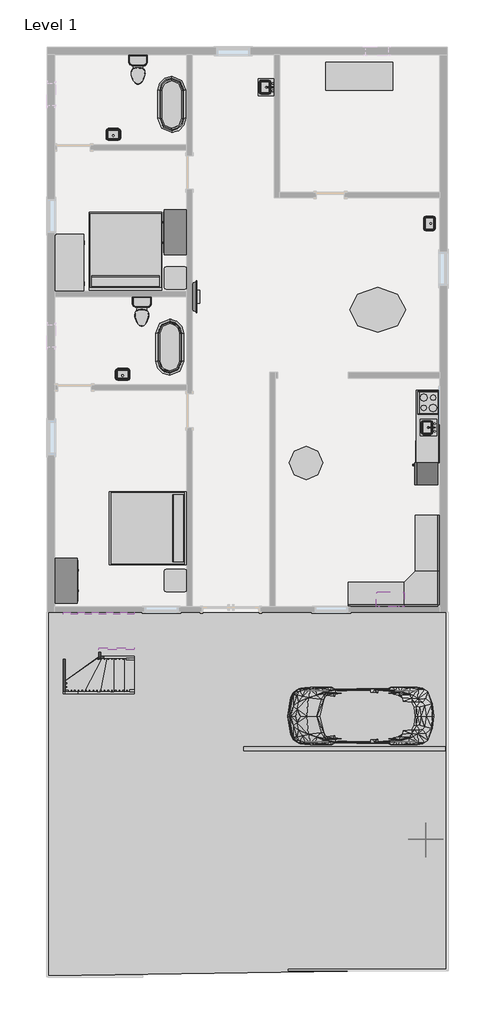
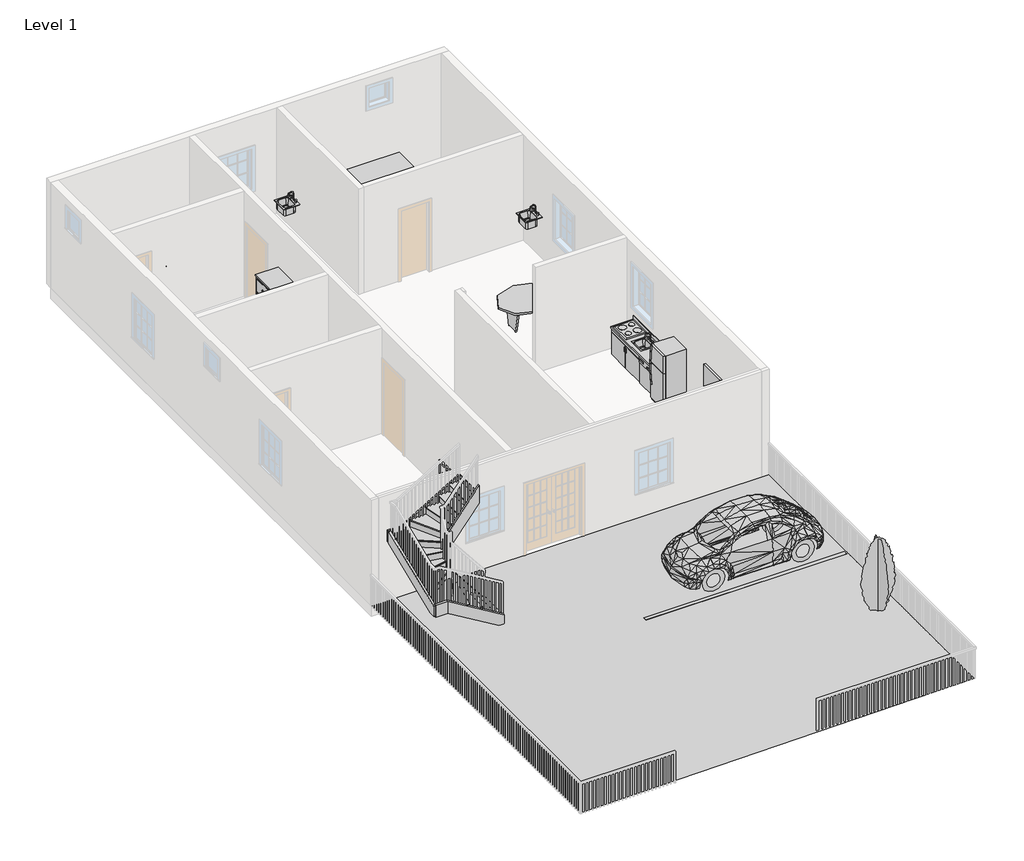
# One storey, part 5 of 5: 13 furniture elements, 9 flow terminals, 8 members, 8 proxies, 1 geographic element, 1 stair flight.
"""IFC4 building model written with IfcOpenShell, lengths in millimetres."""

from ifc_helpers import new_model, si_unit, frame, origin, place, context, project, spatial, polyline, outline, extrude, triangles, transform, mapped, element, save
from components import proxy_a6faaae8, proxy_45b28599, kitchenette_medium_kitchenette_medium_844211aa, proxy_8a8d5ab2, parking_space_9_x_18_90_deg_b8b21359, rpc_beetle_rpc_beetle_3ce7ba48, proxy_c523a7b7, flow_terminal_871c2e40, toilet_domestic_3d_toilet_domestic_3d_f7549cf7, toilet_domestic_3d_toilet_domestic_3d_183bbd19, flow_terminal_b374fae2, flow_terminal_f2f0329d, furniture_29cd36cd, furniture_c6510c7c, furniture_013ab306, furniture_9fa109b2, furniture_56245f3a, furniture_905aceb5, furniture_743965d2, furniture_bcf351fa, furniture_a5b052b6, furniture_45e3acac, rpc_tree_conifer_chinese_juniper_7_1b9786cd, stair_flight_9fd4ca1a

model = new_model("IFC4")

# Units and contexts
model_context = context("Model", 3, world=origin())
ifc_project = project(units=[si_unit("LENGTHUNIT", "METRE", prefix="MILLI")], contexts=[model_context])

# Site, building, storey
site = spatial("IfcSite", under=ifc_project)
building = spatial("IfcBuilding", under=site)
storey = spatial("IfcBuildingStorey", under=building, Name="Level 1", Elevation=0.0)

# Proxies
placement = place(None, origin())
element("IfcBuildingElementProxy", 1, Name="Building Element Proxy", at=placement, inside=storey, context=model_context, shape_type="Tessellation", body=[
    triangles([(-8987.0171402, -2473.4077469, 0.0), (-8987.0171402, -12354.0075531, 0.0), (1849.2579082, -12201.6075531, 0.0), (1833.3830051, -2473.4077469, 0.0)], [[1, 2, 3], [3, 4, 1]], closed=False),
])
proxy_shape = proxy_a6faaae8(model_context)
element("IfcBuildingElementProxy", 2, Name="Cook Top-4 Unit2 : 22\" x 20\"", ObjectType="Cook Top-4 Unit2 : 22\" x 20\"", at=placement, inside=storey, context=model_context, shape_type="MappedRepresentation", body=[
    mapped(proxy_shape, transform((1350.7829734, 3228.8923354, 0.0), x_axis=(0.0, -1.0000000000000004, 0.0), y_axis=(1.0000000000000004, 0.0, 0.0), z_axis=(0.0, 0.0, 1.0))),
])
proxy_2_shape = proxy_45b28599(model_context)
element("IfcBuildingElementProxy", 3, Name="Dishwasher : 24\" x 24\" x 34\"", ObjectType="Dishwasher : 24\" x 24\" x 34\"", at=placement, inside=storey, context=model_context, shape_type="MappedRepresentation", body=[
    mapped(proxy_2_shape, transform((1058.9334086, 2277.7098039, 0.0), x_axis=(0.0, -1.0000000000000004, 0.0), y_axis=(1.0000000000000004, 0.0, 0.0), z_axis=(0.0, 0.0, 1.0))),
])
kitchenette_medium_kitchenette_medium_shape = kitchenette_medium_kitchenette_medium_844211aa(model_context)
element("IfcBuildingElementProxy", 4, Name="Kitchenette - Medium : Kitchenette - Medium", ObjectType="Kitchenette - Medium : Kitchenette - Medium", at=placement, inside=storey, context=model_context, shape_type="MappedRepresentation", body=[
    mapped(kitchenette_medium_kitchenette_medium_shape, transform((1655.5829734, 2904.7300403, 0.0), x_axis=(0.0, -1.0000000000000004, 0.0), y_axis=(1.0000000000000004, 0.0, 0.0), z_axis=(0.0, 0.0, 1.0))),
])
proxy_3_shape = proxy_8a8d5ab2(model_context)
element("IfcBuildingElementProxy", 5, Name="Microwave : 30\" x 16\" x 18\"", ObjectType="Microwave : 30\" x 16\" x 18\"", at=placement, inside=storey, context=model_context, shape_type="MappedRepresentation", body=[
    mapped(proxy_3_shape, transform((-190.9099039, -1764.7271588, 304.8), x_axis=(1.0, 0.0, 0.0), y_axis=(0.0, 1.0, 0.0), z_axis=(0.0, 0.0, 1.0))),
])
parking_space_9_x_18_90_deg_shape = parking_space_9_x_18_90_deg_b8b21359(model_context)
element("IfcBuildingElementProxy", 6, Name="Parking Space : 9' x 18' - 90 deg", ObjectType="Parking Space : 9' x 18' - 90 deg", at=placement, inside=storey, context=model_context, shape_type="MappedRepresentation", body=[
    mapped(parking_space_9_x_18_90_deg_shape, transform((-3678.4170266, -6181.8076646, 0.0), x_axis=(0.0, 1.0, 0.0), y_axis=(-1.0, 0.0, 0.0), z_axis=(0.0, 0.0, 1.0))),
])
rpc_beetle_rpc_beetle_shape = rpc_beetle_rpc_beetle_3ce7ba48(model_context)
element("IfcBuildingElementProxy", 7, Name="RPC Beetle : RPC Beetle", ObjectType="RPC Beetle : RPC Beetle", at=placement, inside=storey, context=model_context, shape_type="MappedRepresentation", body=[
    mapped(rpc_beetle_rpc_beetle_shape, transform((741.1829734, -5292.8076646, 0.0), x_axis=(0.0, 1.0000000000000002, 0.0), y_axis=(-1.0000000000000002, 0.0, 0.0), z_axis=(0.0, 0.0, 1.0))),
])
proxy_4_shape = proxy_c523a7b7(model_context)
element("IfcBuildingElementProxy", 8, Name="Refrigerator : 24\" x 25\" LH", ObjectType="Refrigerator : 24\" x 25\" LH", at=placement, inside=storey, context=model_context, shape_type="MappedRepresentation", body=[
    mapped(proxy_4_shape, transform((1305.1340019, 1292.1423354, 0.0), x_axis=(0.0, -1.0000000000000004, 0.0), y_axis=(1.0000000000000004, 0.0, 0.0), z_axis=(0.0, 0.0, 1.0))),
])

# Flow terminals
flow_terminal_shape = flow_terminal_871c2e40(model_context)
element("IfcFlowTerminal", 9, ObjectType="Sink Kitchen-Island : 18\" x 18\"", at=placement, inside=storey, context=model_context, shape_type="MappedRepresentation", body=[
    mapped(flow_terminal_shape, transform((-7206.027786, 10495.6377365, 304.8), x_axis=(-1.0000000000000004, 0.0, 0.0), y_axis=(0.0, -1.0000000000000004, 0.0), z_axis=(0.0, 0.0, 1.0))),
])
element("IfcFlowTerminal", 10, ObjectType="Sink Kitchen-Island : 18\" x 18\"", at=placement, inside=storey, context=model_context, shape_type="MappedRepresentation", body=[
    mapped(flow_terminal_shape, transform((-6952.027786, 3967.8377365, 304.8), x_axis=(-1.0000000000000002, 0.0, 0.0), y_axis=(0.0, -1.0000000000000002, 0.0), z_axis=(0.0, 0.0, 1.0))),
])
element("IfcFlowTerminal", 11, ObjectType="Sink Kitchen-Island : 18\" x 18\"", at=placement, inside=storey, context=model_context, shape_type="MappedRepresentation", body=[
    mapped(flow_terminal_shape, transform((1348.4375723, 2571.481576, -14.4), x_axis=(0.0, -1.0000000000000004, 0.0), y_axis=(1.0000000000000004, 0.0, 0.0), z_axis=(0.0, 0.0, 1.0))),
])
element("IfcFlowTerminal", 12, ObjectType="Sink Kitchen-Island : 18\" x 18\"", at=placement, inside=storey, context=model_context, shape_type="MappedRepresentation", body=[
    mapped(flow_terminal_shape, transform((1411.9375723, 8121.381576, 304.8), x_axis=(0.0, -1.0000000000000004, 0.0), y_axis=(1.0000000000000004, 0.0, 0.0), z_axis=(0.0, 0.0, 1.0))),
])
element("IfcFlowTerminal", 13, ObjectType="Sink Kitchen-Island : 18\" x 18\"", at=placement, inside=storey, context=model_context, shape_type="MappedRepresentation", body=[
    mapped(flow_terminal_shape, transform((-3058.4624277, 11829.781576, 0.0), x_axis=(0.0, -1.0000000000000002, 0.0), y_axis=(1.0000000000000002, 0.0, 0.0), z_axis=(0.0, 0.0, 1.0))),
])
toilet_domestic_3d_toilet_domestic_3d_shape = toilet_domestic_3d_toilet_domestic_3d_f7549cf7(model_context)
toilet_domestic_3d_toilet_domestic_3d_2_shape = toilet_domestic_3d_toilet_domestic_3d_183bbd19(model_context)
element("IfcFlowTerminal", 14, ObjectType="Toilet-Domestic-3D : Toilet-Domestic-3D", at=placement, inside=storey, context=model_context, shape_type="MappedRepresentation", body=[
    mapped(toilet_domestic_3d_toilet_domestic_3d_shape, transform((-6548.6170266, 12195.6963081, 0.0), x_axis=(1.0, 0.0, 0.0), y_axis=(0.0, 1.0, 0.0), z_axis=(0.0, 0.0, 1.0))),
    mapped(toilet_domestic_3d_toilet_domestic_3d_2_shape, transform((-6548.6170266, 12195.6963081, 0.0), x_axis=(1.0, 0.0, 0.0), y_axis=(0.0, 1.0, 0.0), z_axis=(0.0, 0.0, 1.0))),
])
element("IfcFlowTerminal", 15, ObjectType="Toilet-Domestic-3D : Toilet-Domestic-3D", at=placement, inside=storey, context=model_context, shape_type="MappedRepresentation", body=[
    mapped(toilet_domestic_3d_toilet_domestic_3d_shape, transform((-6447.0170266, 5617.0963081, 0.0), x_axis=(1.0, 0.0, 0.0), y_axis=(0.0, 1.0, 0.0), z_axis=(0.0, 0.0, 1.0))),
    mapped(toilet_domestic_3d_toilet_domestic_3d_2_shape, transform((-6447.0170266, 5617.0963081, 0.0), x_axis=(1.0, 0.0, 0.0), y_axis=(0.0, 1.0, 0.0), z_axis=(0.0, 0.0, 1.0))),
])
flow_terminal_2_shape = flow_terminal_b374fae2(model_context)
element("IfcFlowTerminal", 16, ObjectType="Tub-Free Standing-3D : 30\" x 60\"", at=placement, inside=storey, context=model_context, shape_type="MappedRepresentation", body=[
    mapped(flow_terminal_2_shape, transform((-5685.0170266, 4740.1923354, 0.0), x_axis=(1.0, 0.0, 0.0), y_axis=(0.0, 1.0, 0.0), z_axis=(0.0, 0.0, 1.0))),
])
flow_terminal_3_shape = flow_terminal_f2f0329d(model_context)
element("IfcFlowTerminal", 17, ObjectType="Tub-Free Standing-3D : 30\" x 60\"", at=placement, inside=storey, context=model_context, shape_type="MappedRepresentation", body=[
    mapped(flow_terminal_3_shape, transform((-5634.2170266, 11344.1923354, 0.0), x_axis=(-1.0, 0.0, 0.0), y_axis=(0.0, -1.0, 0.0), z_axis=(0.0, 0.0, 1.0))),
])

# Furniture
furniture_shape = furniture_29cd36cd(model_context)
element("IfcFurniture", 18, ObjectType="Bed-Shaker : King 78\" x 83\"", at=placement, inside=storey, context=model_context, shape_type="MappedRepresentation", body=[
    mapped(furniture_shape, transform((-6907.9645676, 6309.1628272, 0.0), x_axis=(-1.0000000000000002, 0.0, 0.0), y_axis=(0.0, -1.0000000000000002, 0.0), z_axis=(0.0, 0.0, 1.0))),
])
element("IfcFurniture", 19, ObjectType="Bed-Shaker : King 78\" x 83\"", at=placement, inside=storey, context=model_context, shape_type="MappedRepresentation", body=[
    mapped(furniture_shape, transform((-5227.8170266, -206.4576646, 0.0), x_axis=(0.0, -1.0, 0.0), y_axis=(1.0, 0.0, 0.0), z_axis=(0.0, 0.0, 1.0))),
])
furniture_2_shape = furniture_c6510c7c(model_context)
element("IfcFurniture", 20, ObjectType="Counter Top w Sink Hole : 24\" Depth", at=placement, inside=storey, context=model_context, shape_type="MappedRepresentation", body=[
    mapped(furniture_2_shape, transform((1655.5829734, 2371.3300403, -14.4), x_axis=(0.0, -1.0000000000000004, 0.0), y_axis=(1.0000000000000004, 0.0, 0.0), z_axis=(0.0, 0.0, 1.0))),
])
furniture_3_shape = furniture_013ab306(model_context)
element("IfcFurniture", 21, ObjectType="Desk : 60\" x 30\" Student", at=placement, inside=storey, context=model_context, shape_type="MappedRepresentation", body=[
    mapped(furniture_3_shape, transform((-8047.2170266, 6264.1923354, 0.0), x_axis=(0.0, 1.0000000000000002, 0.0), y_axis=(-1.0000000000000002, 0.0, 0.0), z_axis=(0.0, 0.0, 1.0))),
])
furniture_4_shape = furniture_9fa109b2(model_context)
element("IfcFurniture", 22, ObjectType="Dresser : 48\" x 72\" x 24\"", at=placement, inside=storey, context=model_context, shape_type="MappedRepresentation", body=[
    mapped(furniture_4_shape, transform((-5169.4540725, 7595.1990756, 0.0), x_axis=(0.0, -1.0, 0.0), y_axis=(1.0, 0.0, 0.0), z_axis=(0.0, 0.0, 1.0))),
])
element("IfcFurniture", 23, ObjectType="Dresser : 48\" x 72\" x 24\"", at=placement, inside=storey, context=model_context, shape_type="MappedRepresentation", body=[
    mapped(furniture_4_shape, transform((-8867.5799807, -1340.6144047, 0.0), x_axis=(0.0, 1.0, 0.0), y_axis=(-1.0, 0.0, 0.0), z_axis=(0.0, 0.0, 1.0))),
])
furniture_5_shape = furniture_56245f3a(model_context)
element("IfcFurniture", 24, ObjectType="TV - Flat Screen : 32\"", at=placement, inside=storey, context=model_context, shape_type="MappedRepresentation", body=[
    mapped(furniture_5_shape, transform((-5016.8784029, 6115.7368496, 914.4), x_axis=(0.0, 1.0, 0.0), y_axis=(-1.0, 0.0, 0.0), z_axis=(0.0, 0.0, 1.0))),
])
furniture_6_shape = furniture_905aceb5(model_context)
element("IfcFurniture", 25, ObjectType="Table-Dining Round w Chairs : 36\" Diameter", at=placement, inside=storey, context=model_context, shape_type="MappedRepresentation", body=[
    mapped(furniture_6_shape, transform((-2080.2989938, 1775.4710239, 0.0), x_axis=(1.0, 0.0, 0.0), y_axis=(0.0, 1.0, 0.0), z_axis=(0.0, 0.0, 1.0))),
])
furniture_7_shape = furniture_743965d2(model_context)
element("IfcFurniture", 26, ObjectType="Table-Ellipse : 60\" x 48\"", at=placement, inside=storey, context=model_context, shape_type="MappedRepresentation", body=[
    mapped(furniture_7_shape, transform((-33.5170266, 5756.1923354, 0.0), x_axis=(1.0, 0.0, 0.0), y_axis=(0.0, 1.0, 0.0), z_axis=(0.0, 0.0, 1.0))),
])
furniture_8_shape = furniture_bcf351fa(model_context)
element("IfcFurniture", 27, ObjectType="Table-End : 24\" x 24\"", at=placement, inside=storey, context=model_context, shape_type="MappedRepresentation", body=[
    mapped(furniture_8_shape, transform((-5841.1506569, 6467.3923354, 0.0), x_axis=(1.0, 0.0, 0.0), y_axis=(0.0, 1.0, 0.0), z_axis=(0.0, 0.0, 1.0))),
])
element("IfcFurniture", 28, ObjectType="Table-End : 24\" x 24\"", at=placement, inside=storey, context=model_context, shape_type="MappedRepresentation", body=[
    mapped(furniture_8_shape, transform((-5841.1506569, -1762.2076646, 0.0), x_axis=(1.0, 0.0, 0.0), y_axis=(0.0, 1.0, 0.0), z_axis=(0.0, 0.0, 1.0))),
])
furniture_9_shape = furniture_a5b052b6(model_context)
element("IfcFurniture", 29, ObjectType="Table-Rectangular : 72\" x 30\"", at=placement, inside=storey, context=model_context, shape_type="MappedRepresentation", body=[
    mapped(furniture_9_shape, transform((-528.8170266, 12106.1923354, 0.0), x_axis=(1.0, 0.0, 0.0), y_axis=(0.0, 1.0, 0.0), z_axis=(0.0, 0.0, 1.0))),
])
furniture_10_shape = furniture_45e3acac(model_context)
element("IfcFurniture", 30, ObjectType="Work Station Cubicle : 96\" x 96\"", at=placement, inside=storey, context=model_context, shape_type="MappedRepresentation", body=[
    mapped(furniture_10_shape, transform((1523.8512212, -2816.0306722, 0.0), x_axis=(-1.0000000000000004, 0.0, 0.0), y_axis=(0.0, -1.0000000000000004, 0.0), z_axis=(0.0, 0.0, 1.0))),
])

# Geographic element
rpc_tree_conifer_chinese_juniper_7_shape = rpc_tree_conifer_chinese_juniper_7_1b9786cd(model_context)
element("IfcGeographicElement", 31, ObjectType="RPC Tree - Conifer : Chinese Juniper - 7'", at=placement, inside=storey, context=model_context, shape_type="MappedRepresentation", body=[
    mapped(rpc_tree_conifer_chinese_juniper_7_shape, transform((1274.3863024, -8645.6076646, 0.0), x_axis=(1.0, 0.0, 0.0), y_axis=(0.0, 1.0, 0.0), z_axis=(0.0, 0.0, 1.0))),
])

# Members
element("IfcMember", 32, ObjectType="Stringer - 2\" Width", at=placement, inside=storey, context=model_context, shape_type="SweptSolid", body=[
    extrude(outline(polyline([(0.0, -6646.4853347), (261.162507, -6646.4853347), (1192.0522894, -8191.5788955), (836.2077775, -8191.5788955), (0.0, -6803.638801), (0.0, -6646.4853347)])), frame((0.0, -4683.2076646, 0.0), z_axis=(0.0, 1.0, 0.0), x_axis=(0.0, 0.0, 1.0)), (0.0, 0.0, 1.0), 50.8),
])
element("IfcMember", 33, ObjectType="Stringer - 2\" Width", at=placement, inside=storey, context=model_context, shape_type="SweptSolid", body=[
    extrude(outline(polyline([(-8191.5788955, -4632.4076646), (-8191.5788955, -4683.2076646), (-8529.8170266, -4683.2076646), (-8529.8170266, -4632.4076646), (-8191.5788955, -4632.4076646)])), frame((0.0, 0.0, 836.2077775), z_axis=(0.0, 0.0, 1.0), x_axis=(1.0, 0.0, 0.0)), (0.0, 0.0, 1.0), 355.8445119),
])
element("IfcMember", 34, ObjectType="Stringer - 2\" Width", at=placement, inside=storey, context=model_context, shape_type="SweptSolid", body=[
    extrude(outline(polyline([(-4683.2076646, 887.2522894), (-4683.2076646, 1171.0946013), (-2559.7227754, 2047.144485), (-2524.2076646, 2047.144485), (-2524.2076646, 1705.9518356), (-4508.6792654, 887.2522894), (-4683.2076646, 887.2522894)])), frame((-8580.6170266, 0.0, 0.0), z_axis=(1.0, 0.0, 0.0), x_axis=(0.0, 1.0, 0.0)), (0.0, 0.0, 1.0), 50.8),
])
element("IfcMember", 35, ObjectType="Stringer - 2\" Width", at=placement, inside=storey, context=model_context, shape_type="SweptSolid", body=[
    extrude(outline(polyline([(-8580.6170266, -2524.2076646), (-8580.6170266, -2473.4076646), (-8191.5788955, -2473.4076646), (-8191.5788955, -2524.2076646), (-8580.6170266, -2524.2076646)])), frame((0.0, 0.0, 1717.4247116), z_axis=(0.0, 0.0, 1.0), x_axis=(1.0, 0.0, 0.0)), (0.0, 0.0, 1.0), 329.7197733),
])
element("IfcMember", 36, ObjectType="Stringer - 2\" Width", at=placement, inside=storey, context=model_context, shape_type="SweptSolid", body=[
    extrude(outline(polyline([(2047.144485, -8191.5788955), (1717.4247116, -8191.5788955), (2648.314494, -6646.4853347), (2978.0342674, -6646.4853347), (2047.144485, -8191.5788955)])), frame((0.0, -2524.2076646, 0.0), z_axis=(0.0, 1.0, 0.0), x_axis=(0.0, 0.0, 1.0)), (0.0, 0.0, 1.0), 50.8),
])
element("IfcMember", 37, ObjectType="Stringer - 2\" Width", at=placement, inside=storey, context=model_context, shape_type="SweptSolid", body=[
    extrude(outline(polyline([(0.0, -6646.4853347), (162.1507007, -6646.4853347), (1325.54903, -7564.6170266), (833.5414661, -7564.6170266), (0.0, -6906.802057), (0.0, -6646.4853347)])), frame((0.0, -3718.0076646, 0.0), z_axis=(0.0, 1.0, 0.0), x_axis=(0.0, 0.0, 1.0)), (0.0, 0.0, 1.0), 50.8),
])
element("IfcMember", 38, ObjectType="Stringer - 2\" Width", at=placement, inside=storey, context=model_context, shape_type="SweptSolid", body=[
    extrude(outline(polyline([(-3718.0076646, 897.9120087), (-3718.0076646, 1570.0688755), (-3505.1979288, 2037.3149397), (-3489.4076646, 2037.3149397), (-3489.4076646, 1336.621023), (-3689.2200473, 897.9120087), (-3718.0076646, 897.9120087)])), frame((-7615.4170266, 0.0, 0.0), z_axis=(1.0, 0.0, 0.0), x_axis=(0.0, 1.0, 0.0)), (0.0, 0.0, 1.0), 50.8),
])
element("IfcMember", 39, ObjectType="Stringer - 2\" Width", at=placement, inside=storey, context=model_context, shape_type="SweptSolid", body=[
    extrude(outline(polyline([(2037.3149397, -7615.4170266), (1545.3073758, -7615.4170266), (2773.0762477, -6646.4853347), (3265.0838115, -6646.4853347), (2037.3149397, -7615.4170266)])), frame((0.0, -3489.4076646, 0.0), z_axis=(0.0, 1.0, 0.0), x_axis=(0.0, 0.0, 1.0)), (0.0, 0.0, 1.0), 50.8),
])

# Stair flight
stair_flight_shape = stair_flight_9fd4ca1a(model_context)
element("IfcStairFlight", 40, ObjectType="2\" Tread 1\" Nosing 1/4\" Riser", at=placement, inside=storey, context=model_context, shape_type="MappedRepresentation", body=[
    mapped(stair_flight_shape, transform((0.0, 0.0, 0.0), x_axis=(1.0, 0.0, 0.0), y_axis=(0.0, 1.0, 0.0), z_axis=(0.0, 0.0, 1.0))),
])

save(model, "model.ifc")

# Revit data of these elements
# Type "Cook Top-4 Unit2 : 22\" x 20\""
#   Depth = 1' - 8"
#   Width = 1' - 10"
#   Burner Material = Steel, Chrome Plated
#   Cooktop Material = Steel, Polished
#   Default Elevation = 0
#   Assembly Code = ""
# Type "Dishwasher : 24\" x 24\" x 34\""
#   Label = "DW"
#   Assembly Code = "E1090400"
#   Depth = 2' - 0"
#   Height = 2' - 10"
#   Width = 2' - 0"
#   Dishwasher Material = Steel, Paint Finish, Ivory, Glossy
#   Panel Face Material = Plastic, Opaque Black
#   Default Elevation = 0
# Type "Kitchenette - Medium : Kitchenette - Medium"
#   Assembly Code = "E1090400"
#   Counter Length = 6' - 6"
#   Cabinet Width = 4' - 6"
#   Cabinet Height = 2' - 10 1/2"
#   Cabinet Depth = 2' - 0"
#   Toe Depth = 0' - 3"
#   Toe Height = 0' - 3 1/2"
#   Cabinet Material = Cabinets
#   Door/Drawer Material = Cabinets
#   Handle Material = Cabinets - Handles
#   Default Elevation = 0
# Type "Microwave : 30\" x 16\" x 18\""
#   Assembly Code = "E1090400"
#   Depth = 1' - 4"
#   Height = 1' - 6"
#   Width = 2' - 6"
#   Microwave Material = Laminate, Ivory, Matte
#   Default Elevation = 0
# Type "Parking Space : 9' x 18' - 90 deg"
#   Angle = 90.00°
#   Parking Length = 18' - 0"
#   Parking Width = 9' - 0"
#   pl = 18' - 0"
#   pw = 9' - 0"
# Type "RPC Beetle : RPC Beetle"
#   built-in parameter 1005195 = "RPC-16-0U6E-L4EG-ENH1-J3KF-SVEL-0TX4-C0"
#   Height = 0
# Type "Refrigerator : 24\" x 25\" LH"
#   Label = "REF."
#   Assembly Code = "E1090400"
#   Depth = 2' - 0 3/4"
#   Handle = 0' - 1 1/2"
#   Height = 5' - 3 1/2"
#   Rear Clearance = 0' - 2"
#   Top Door Height = 1' - 8"
#   Width = 1' - 11 1/2"
#   Material = Steel, Paint Finish, Ivory, Glossy
#   Default Elevation = 0
# Type "Sink Kitchen-Island : 18\" x 18\""
#   Assembly Code = "D2010410"
#   Counter Height = 3' - 0"
#   Depth = 1' - 6"
#   Width = 1' - 6"
#   Faucet Material = Steel, Polished
#   Sink Material = Steel, Polished
#   Default Elevation = 0
# Type "Toilet-Domestic-3D : Toilet-Domestic-3D"
#   Assembly Code = "D2010110"
#   Toilet - Bowl/Basin Material = Porcelain, Linen
#   Toilet - Seat Material = Laminate, Linen, Matte
#   Default Elevation = 0
# Type "Tub-Free Standing-3D : 30\" x 60\""
#   Assembly Code = "D2010110"
#   Height = 1' - 6"
#   Length = 5' - 0"
#   Width = 2' - 6"
#   Tub Material = Porcelain, Ivory
#   Default Elevation = 0
# Type "Bed-Shaker : King 78\" x 83\""
#   Assembly Code = "E2020200"
#   Length = 6' - 11"
#   Width = 6' - 6"
#   Frame Material = Birch
#   Mattress Material = Linen, White
#   Default Elevation = 0
# Type "Counter Top w Sink Hole : 24\" Depth"
#   Assembly Code = "C1030400"
#   Counter Thickness = 0' - 1 1/2"
#   Depth [instance default] = 2' - 1"
#   Height = 3' - 0"
#   Length [instance default] = 8' - 0"
#   Sink Location [instance default] = 2' - 0"
#   Sink Location To Wall [instance default] = 0' - 6"
#   Sink Opening Depth [instance default] = 1' - 3"
#   Sink Opening Width [instance default] = 2' - 3"
#   Counter Top Material = none
#   Default Elevation = 0
# Type "Desk : 60\" x 30\" Student"
#   Assembly Code = "E2020200"
#   Depth = 2' - 6"
#   Height = 2' - 6"
#   Leg Height = 0' - 6"
#   Width = 5' - 0"
#   Body Material = Laminate, Ivory, Matte
#   Handle/Leg Material = Steel, Chrome Plated
#   Top Material = Cherry
#   Default Elevation = 0
# Type "Dresser : 48\" x 72\" x 24\""
#   Assembly Code = "E2020200"
#   Depth = 2' - 0"
#   Height = 6' - 0"
#   Width = 4' - 0"
#   Dresser Material = Laminate - Ivory, Glossy
#   Drawer Material = Laminate, Ivory, Matte
#   Knob Material = Cherry
#   Default Elevation = 0
# Type "TV - Flat Screen : 32\""
#   SinAng = 0' - 0.0193"
#   L = 2' - 3.79372"
#   H = 1' - 3.6354"
#   Thickness = 0' - 4.33071"
#   Diagonal = 2' - 7.88976"
#   CosAng = 0' - 0.03431"
#   Stand [instance default] = yes
#   Default Elevation = 0
# Type "Table-Dining Round w Chairs : 36\" Diameter"
#   Assembly Code = "E2020200"
#   Radius = 1' - 6"
#   Diameter = 3' - 0"
#   Height = 2' - 6"
#   Chairs = 4
#   Base Material = Pine
#   Top Material = Laminate, Linen, Matte
#   Default Elevation = 0
# Type "Table-Ellipse : 60\" x 48\""
#   Assembly Code = "E2020200"
#   Half Width = 2' - 0"
#   Half Length = 2' - 6"
#   Height = 2' - 6"
#   Length = 5' - 0"
#   Width = 4' - 0"
#   Base Material = Birch
#   Top Material = Birch
#   Default Elevation = 0
# Type "Table-End : 24\" x 24\""
#   Assembly Code = "E2020200"
#   Height = 2' - 6"
#   Length = 2' - 0"
#   Width = 2' - 0"
#   Base Material = Birch
#   Top Material = Laminate, Ivory, Matte
#   Default Elevation = 0
# Type "Table-Rectangular : 72\" x 30\""
#   Assembly Code = "E2020200"
#   Height = 2' - 6"
#   Length = 6' - 0"
#   Width = 2' - 6"
#   Base Material = Birch
#   Top Material = Birch
#   Default Elevation = 0
# Type "Work Station Cubicle : 96\" x 96\""
#   Assembly Code = "E2020"
#   Desktop Height = 2' - 6"
#   Desktop1 Width = 2' - 0"
#   Desktop2 Width = 2' - 0"
#   Panel Height = 5' - 6"
#   Panel1 Length = 5' - 0"
#   Panel2 Length = 5' - 0"
#   Cube Panel Material = Textile - Light Gray
#   Work Top Material = Laminate, Ivory, Matte
#   Default Elevation = 0
# Type "RPC Tree - Conifer : Chinese Juniper - 7'"
#   built-in parameter 1005198 = "{2, 15},{39, RPC-16-FUM3-UUQ0-UBF0-N000-ST1L-LVER-AU},{1, 0},{1, 0},{2, 13},{1, 8},{5, Color},{1, 0},{1, 0},{3, 0.8},{3, 0.8},{3, 0.8},{1, 8},{7, BBoxMin},{1, 0},{1, 0},{1, 0},{1, 0},{1, 0},{1, 8},{7, BBoxMax},{1, 0},{1, 0},{1, 0},{1, 0},{1, 0},{2, 11},{9, RPCTypeId},{1, 0},{1, 0},{39, RPC-16-FUM3-UUQ0-UBF0-N000-ST1L-LVER-AU},{1, 6},{14, RPCPlantHeight},{1, 0},{1, 0},{1, 7},{2, 11},{7, keyword},{1, 0},{1, 0},{34, :RPCs:Trees [General]:Geometry:RPC},{2, 11},{8, category},{1, 0},{1, 0},{15, Trees [General]},{2, 11},{12, LocalizedUID},{1, 0},{1, 0},{15, Chinese Juniper},{2, 14},{6, Height},{1, 0},{1, 0},{1, 7},{1, 2},{16, Cast Reflections},{1, 0},{1, 0},{1, 0},{1, 2},{12, Cast Shadows},{1, 0},{1, 0},{1, 1},{1, 2},{9, Lock View},{1, 0},{1, 0},{1, 0},{1, 4},{5, ViewC},{1, 0},{1, 0},{1, 0},{21, assetlibrary_base.fbx},{1, 5},"
#   built-in parameter 1005195 = "RPC-16-FUM3-UUQ0-UBF0-N000-ST1L-LVER-AU"
#   Type Comments = "Chinese Juniper"
#   Assembly Code = "G2050500"
#   Height = 7' - 0"
#   Description = (empty or 0)
#   Default Elevation = 0
# Element 1 (IfcBuildingElementProxy)
#   Material = none
#   Phase Created = New Construction
# Element 2 (IfcBuildingElementProxy, "Cook Top-4 Unit2 : 22\" x 20\"")
#   Phase Created = New Construction
#   Materials on its faces: "Steel, Chrome Plated", "Steel, Polished"
# Element 3 (IfcBuildingElementProxy, "Dishwasher : 24\" x 24\" x 34\"")
#   Phase Created = New Construction
#   Materials on its faces: "Steel, Paint Finish, Ivory, Glossy", "Plastic, Opaque Black"
# Element 4 (IfcBuildingElementProxy, "Kitchenette - Medium : Kitchenette - Medium")
#   Phase Created = New Construction
#   Materials on its faces: "Cabinets", "Cabinets - Handles"
# Element 5 (IfcBuildingElementProxy, "Microwave : 30\" x 16\" x 18\"")
#   Phase Created = New Construction
#   Materials on its faces: "Laminate, Ivory, Matte", "Glass"
# Element 6 (IfcBuildingElementProxy, "Parking Space : 9' x 18' - 90 deg")
#   Phase Created = New Construction
#   Materials on its faces: "Parking Stripe"
# Element 7 (IfcBuildingElementProxy, "RPC Beetle : RPC Beetle")
#   Phase Created = New Construction
# Element 8 (IfcBuildingElementProxy, "Refrigerator : 24\" x 25\" LH")
#   Phase Created = New Construction
#   Materials on its faces: "Steel, Paint Finish, Ivory, Glossy", "Steel, Chrome Plated"
# Element 9 (IfcFlowTerminal, "Sink Kitchen-Island : 18\" x 18\"")
#   Mark = "3"
#   Phase Created = New Construction
#   Materials on its faces: "Steel, Polished"
# Element 10 (IfcFlowTerminal, "Sink Kitchen-Island : 18\" x 18\"")
#   Mark = "6"
#   Phase Created = New Construction
#   Materials on its faces: "Steel, Polished"
# Element 11 (IfcFlowTerminal, "Sink Kitchen-Island : 18\" x 18\"")
#   Mark = "8"
#   Phase Created = New Construction
#   Materials on its faces: "Steel, Polished"
# Element 12 (IfcFlowTerminal, "Sink Kitchen-Island : 18\" x 18\"")
#   Mark = "9"
#   Phase Created = New Construction
#   Materials on its faces: "Steel, Polished"
# Element 13 (IfcFlowTerminal, "Sink Kitchen-Island : 18\" x 18\"")
#   Mark = "20"
#   Phase Created = New Construction
#   Materials on its faces: "Steel, Polished"
# Element 14 (IfcFlowTerminal, "Toilet-Domestic-3D : Toilet-Domestic-3D")
#   Mark = "2"
#   Phase Created = New Construction
#   Materials on its faces: "Porcelain, Linen", "Laminate, Linen, Matte"
# Element 15 (IfcFlowTerminal, "Toilet-Domestic-3D : Toilet-Domestic-3D")
#   Mark = "7"
#   Phase Created = New Construction
#   Materials on its faces: "Porcelain, Linen", "Laminate, Linen, Matte"
# Element 16 (IfcFlowTerminal, "Tub-Free Standing-3D : 30\" x 60\"")
#   Mark = "5"
#   Phase Created = New Construction
#   Materials on its faces: "Porcelain, Ivory"
# Element 17 (IfcFlowTerminal, "Tub-Free Standing-3D : 30\" x 60\"")
#   Mark = "1"
#   Phase Created = New Construction
#   Materials on its faces: "Porcelain, Ivory"
# Elements 18, 19 (IfcFurniture, "Bed-Shaker : King 78\" x 83\"")
#   Phase Created = New Construction
#   Materials on its faces: "Birch", "Linen, White"
# Element 20 (IfcFurniture, "Counter Top w Sink Hole : 24\" Depth")
#   Sink Opening Depth = 1' - 2"
#   Sink Location To Wall = 0' - 6"
#   Length = 6' - 6"
#   Sink Location = 3' - 4"
#   Sink Opening Width = 1' - 4"
#   Phase Created = New Construction
#   Materials on its faces: "Counter Top"
# Element 21 (IfcFurniture, "Desk : 60\" x 30\" Student")
#   Phase Created = New Construction
#   Materials on its faces: "Steel, Chrome Plated", "Laminate, Ivory, Matte", "Cherry"
# Elements 22, 23 (IfcFurniture, "Dresser : 48\" x 72\" x 24\"")
#   Phase Created = New Construction
#   Materials on its faces: "Laminate, Ivory, Matte", "Cherry", "Laminate - Ivory, Glossy"
# Element 24 (IfcFurniture, "TV - Flat Screen : 32\"")
#   Stand = yes
#   Phase Created = New Construction
#   Materials on its faces: "TV - Black", "TV - Glass", "TV - Screen"
# Element 25 (IfcFurniture, "Table-Dining Round w Chairs : 36\" Diameter")
#   Phase Created = New Construction
#   Materials on its faces: "Pine", "Laminate, Linen, Matte"
# Element 26 (IfcFurniture, "Table-Ellipse : 60\" x 48\"")
#   Phase Created = New Construction
#   Materials on its faces: "Birch"
# Elements 27, 28 (IfcFurniture, "Table-End : 24\" x 24\"")
#   Phase Created = New Construction
#   Materials on its faces: "Laminate, Ivory, Matte", "Birch"
# Element 29 (IfcFurniture, "Table-Rectangular : 72\" x 30\"")
#   Phase Created = New Construction
#   Materials on its faces: "Birch"
# Element 30 (IfcFurniture, "Work Station Cubicle : 96\" x 96\"")
#   Phase Created = New Construction
#   Materials on its faces: "Textile - Light Gray", "Laminate, Ivory, Matte"
# Element 31 (IfcGeographicElement, "RPC Tree - Conifer : Chinese Juniper - 7'")
#   Phase Created = New Construction
# Elements 32, 33, 34, 35, 36, 37, 38, 39 (IfcMember, "Stringer - 2\" Width")
#   Phase Created = New Construction
# Element 40 (IfcStairFlight, "2\" Tread 1\" Nosing 1/4\" Riser")
#   Phase Created = New Construction
# Materials
#   "Steel, Chrome Plated": class "Metal", colour RGB 17 17 17, transparency 0, Description = "Chromiuim plated steel", Cost = 0
#   "Steel, Polished": class "Metal", colour RGB 57 57 57, transparency 0, Description = "Polished steel", Cost = 0
#   "Steel, Paint Finish, Ivory, Glossy": class "Metal", colour RGB 247 247 239, transparency 0, Description = "Steel, paint finish, ivory, glossy", Cost = 0
#   "Plastic, Opaque Black": class "Plastic", colour RGB 0 0 0, transparency 0.7, Description = "Plastic, generic, opaque black", Cost = 0
#   "Cabinets": colour RGB 249 249 249, transparency 0
#   "Cabinets - Handles": class "Metal", colour RGB 57 57 57, transparency 0
#   "Laminate, Ivory, Matte": class "Plastic", colour RGB 247 247 239, transparency 0, Description = "Plastic Laminate - Ivory, Matte", Cost = 0
#   "Porcelain, Linen": class "Ceramic", colour RGB 249 239 230, transparency 0, Description = "Porcelain, linen", Cost = 0
#   "Laminate, Linen, Matte": class "Plastic", colour RGB 249 239 230, transparency 0, Description = "Plastic Laminate - Linen, Matte", Cost = 0
#   "Porcelain, Ivory": class "Ceramic", colour RGB 247 247 239, transparency 0, Description = "Porcelain, ivory", Cost = 0
#   "Birch": class "Wood", colour RGB 224 178 126, transparency 0, Description = "Betula Alleghaniensis", Cost = 0
#   "Linen, White": class "Textile", colour RGB 247 247 239, transparency 0, Description = "Linen, white", Cost = 0
#   "Cherry": class "Wood", colour RGB 226 177 128, transparency 0, Description = "Prunus Serotina", Cost = 0
#   "Laminate - Ivory, Glossy": colour RGB 247 247 239, transparency 0
#   "Pine": class "Wood", colour RGB 223 192 134, transparency 0, Description = "Pinus Echinata", Cost = 0
#   "Textile - Light Gray": class "Fabric", colour RGB 204 204 204, transparency 0
#   "Glass": class "Glass", colour RGB 0 128 192, transparency 0.75, Description = "Soda Lime Glass", Cost = 0
#   "Parking Stripe": class "Paint", colour RGB 250 250 91, transparency 0
#   "Counter Top": class "Wood", colour RGB 226 177 128, transparency 0
#   "TV - Black": colour RGB 49 49 49, transparency 0
#   "TV - Glass": colour RGB 157 157 157, transparency 0.9
#   "TV - Screen": colour RGB 0 0 0, transparency 0
